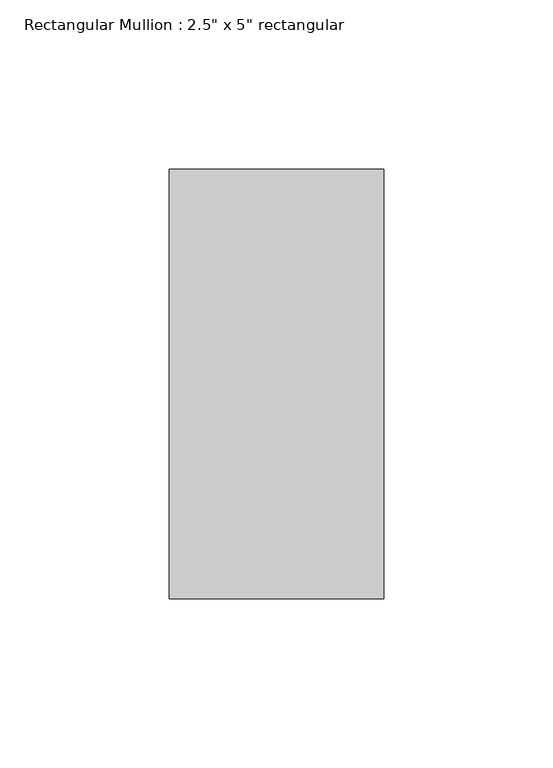
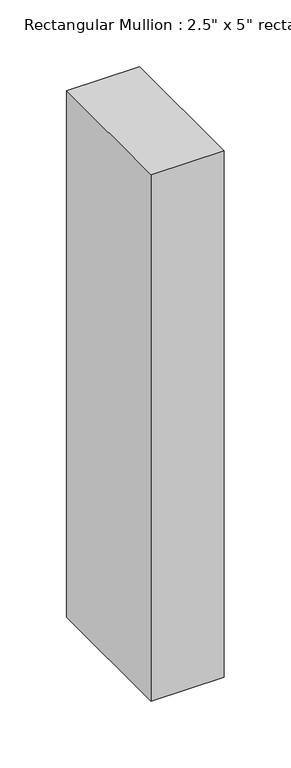
"""IFC4 building model written with IfcOpenShell, lengths in millimetres: member geometry."""

from ifc_helpers import new_model, si_unit, frame, origin, place, context, project, spatial, polyline, outline, extrude, source, transform, mapped, element, save


def member_323df77c(model_context):
    return source(origin(), model_context, "Body", "SweptSolid", [
        extrude(outline(polyline([(31.75, 63.5), (31.75, -63.5), (-31.75, -63.5), (-31.75, 63.5), (31.75, 63.5)])), frame((0.0, 0.0, -482.6), z_axis=(0.0, 0.0, 1.0), x_axis=(1.0, 0.0, 0.0)), (0.0, 0.0, 1.0), 482.6),
    ])


if __name__ == "__main__":
    model = new_model("IFC4")
    model_context = context("Model", 3, world=origin())
    ifc_project = project(units=[si_unit("LENGTHUNIT", "METRE", prefix="MILLI")], contexts=[model_context])
    site = spatial("IfcSite", under=ifc_project)
    building = spatial("IfcBuilding", under=site)
    placement = place(None, origin())
    member_shape = member_323df77c(model_context)
    element("IfcMember", 1, ObjectType="Rectangular Mullion : 2.5\" x 5\" rectangular", at=placement, inside=building, context=model_context, shape_type="MappedRepresentation", body=[
        mapped(member_shape, transform((0.0, 0.0, 0.0), x_axis=(1.0, 0.0, 0.0), y_axis=(0.0, 1.0, 0.0), z_axis=(0.0, 0.0, 1.0))),
    ])
    save(model, "model.ifc")

# Revit data of these elements
# Type "Rectangular Mullion : 2.5\" x 5\" rectangular"
#   built-in parameter 1007304 = 0.416667 (stored number, unit not read)
#   built-in parameter 1007301 = 0.104167 (stored number, unit not read)
#   built-in parameter 1007300 = 0.104167 (stored number, unit not read)
# Element 1 (IfcMember, "Rectangular Mullion : 2.5\" x 5\" rectangular")
#   Materials on its faces: "Rectangle 1 sq"
# Materials
#   "Rectangle 1 sq": class "Generic", colour RGB 120 120 120, transparency 0, Cost = 0
